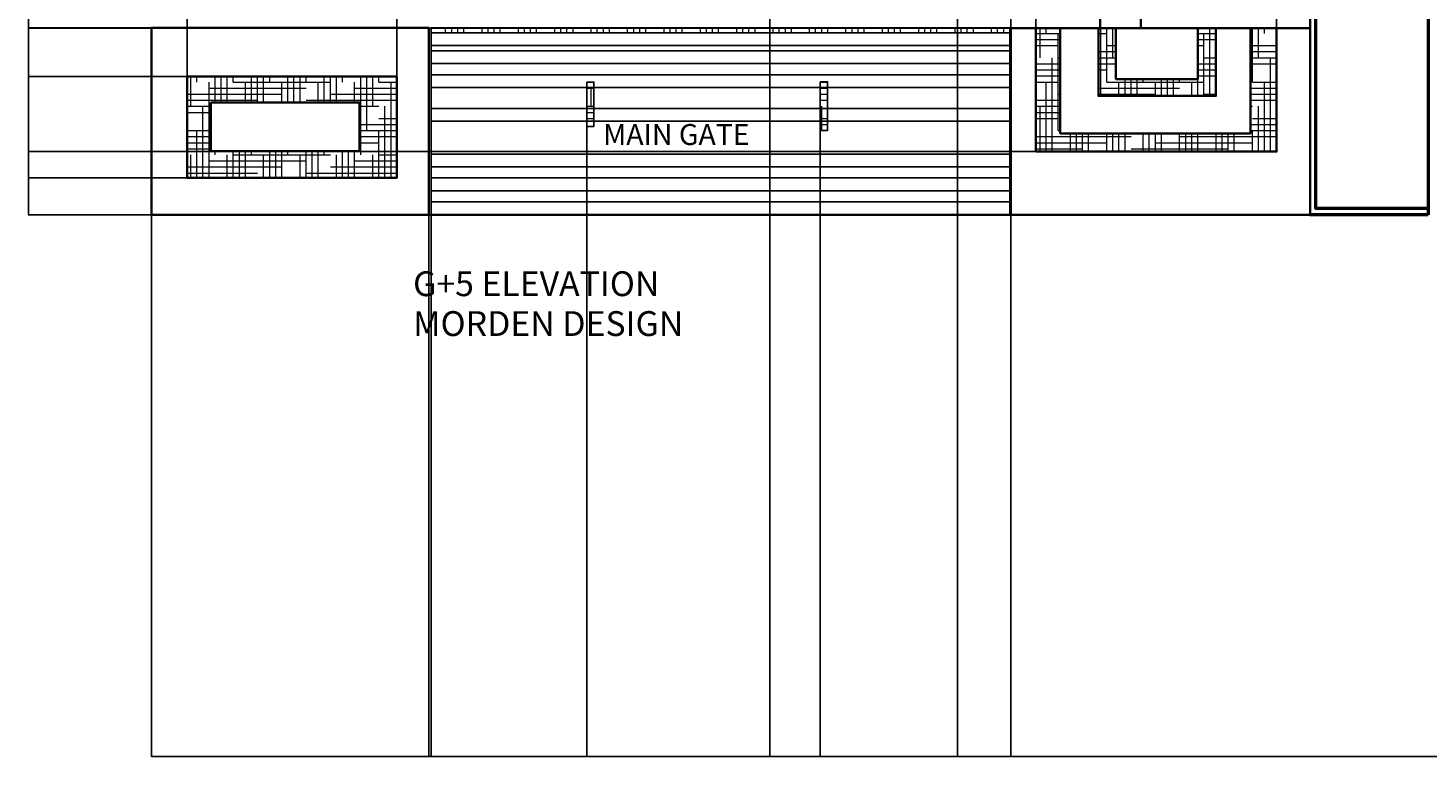
# Model space of a CAD drawing. Units: inches. Extents: x -97 to 1206, y -378 to 680.
# Tile 1 of 6: x -97 to 581, y -378 to -25. Entities that reach past the tile are written whole.
import ezdxf

# ---------------------------------------------------------------- set-up
doc = ezdxf.new("R2010")
doc.units = ezdxf.units.IN
doc.header["$MEASUREMENT"] = 0
for name, color, linetype, lineweight in [('A-ANNO-DIMS', 2, 'Continuous', 18), ('A-ANNO-TEXT', 7, 'Continuous', 25), ('A-DOOR', 3, 'Continuous', 25), ('A-ELEV', 7, 'Continuous', 35), ('A-ELEV-PATT', 252, 'Continuous', 13), ('A-WALL', 7, 'Continuous', 50)]:
    doc.layers.add(name, color=color, linetype=linetype, lineweight=lineweight)
doc.styles.get("Standard").update_dxf_attribs({"font": 'arial.ttf'})
doc.dimstyles.get("Standard").update_dxf_attribs({"dimtxt": 0.18, "dimasz": 0.18, "dimexe": 0.18, "dimexo": 0.0625, "dimgap": 0.09, "dimtad": 0, "dimtih": 1, "dimtoh": 1, "dimdec": 4, "dimzin": 0, "dimdsep": 46, "dimtxsty": 'Standard', "dimcen": 0.09, "dimadec": 0, "dimazin": 0, "dimtfac": 1, "dimtdec": 4, "dimtofl": 0, "dimtmove": 0, "dimatfit": 3, "dimfxl": 1, "dimtolj": 1, "dimtzin": 0, "dimarcsym": 0})

# ---------------------------------------------------------------- blocks, each defined once
blk = doc.blocks.new('*D11')
at = {"layer": 'A-ANNO-DIMS', "color": 0, "lineweight": -2, "transparency": 16777216}
for p, q in [((-36.91, -115.21), (-36.91, -377.59)), ((620.19, -115.21), (620.19, -377.59)), ((-36.73, -377.41), (291.26, -377.41)), ((620.01, -377.41), (292.02, -377.41))]:
    blk.add_line(p, q, dxfattribs=at)
at = {"layer": 'A-ANNO-DIMS', "color": 0, "transparency": 16777216}
for points in [[(-36.73, -377.38), (-36.73, -377.44), (-36.91, -377.41)], [(620.01, -377.38), (620.01, -377.44), (620.19, -377.41)]]:
    blk.add_solid(points, dxfattribs=at)
at = {"layer": 'Defpoints', "color": 0, "transparency": 16777216}
for p in [(-36.91, -115.14), (620.19, -115.14), (620.19, -377.41)]:
    blk.add_point(p, dxfattribs=at)
at = {"layer": 'A-ANNO-DIMS', "color": 0, "transparency": 16777216, "insert": (291.64, -377.41), "char_height": 0.18, "attachment_point": 5}
blk.add_mtext('\\A1;657.1', dxfattribs=at)
blk = doc.blocks.new('*D12')
at = {"layer": 'A-ANNO-DIMS', "color": 0, "lineweight": -2, "transparency": 16777216}
for p, q in [((43.86, 619.86), (-96.59, 619.86)), ((-96.41, 619.68), (-96.41, 252.54)), ((-96.41, -114.96), (-96.41, 252.17)), ((-36.97, -115.14), (-96.59, -115.14))]:
    blk.add_line(p, q, dxfattribs=at)
at = {"layer": 'A-ANNO-DIMS', "color": 0, "transparency": 16777216}
for points in [[(-96.44, 619.68), (-96.38, 619.68), (-96.41, 619.86)], [(-96.44, -114.96), (-96.38, -114.96), (-96.41, -115.14)]]:
    blk.add_solid(points, dxfattribs=at)
at = {"layer": 'Defpoints', "color": 0, "transparency": 16777216}
for p in [(43.93, 619.86), (-96.41, -115.14), (-36.91, -115.14)]:
    blk.add_point(p, dxfattribs=at)
at = {"layer": 'A-ANNO-DIMS', "color": 0, "transparency": 16777216, "insert": (-96.41, 252.36), "char_height": 0.18, "attachment_point": 5}
blk.add_mtext('\\A1;735', dxfattribs=at)
blk = doc.blocks.new('*D13')
at = {"layer": 'A-ANNO-DIMS', "color": 0, "lineweight": -2, "transparency": 16777216}
for p, q in [((46.86, 4.86), (-96.59, 4.86)), ((-96.41, 4.68), (-96.41, -54.96)), ((-96.41, -114.96), (-96.41, -55.33)), ((-36.97, -115.14), (-96.59, -115.14))]:
    blk.add_line(p, q, dxfattribs=at)
at = {"layer": 'A-ANNO-DIMS', "color": 0, "transparency": 16777216}
for points in [[(-96.44, 4.68), (-96.38, 4.68), (-96.41, 4.86)], [(-96.44, -114.96), (-96.38, -114.96), (-96.41, -115.14)]]:
    blk.add_solid(points, dxfattribs=at)
at = {"layer": 'Defpoints', "color": 0, "transparency": 16777216}
for p in [(46.93, 4.86), (-96.41, -115.14), (-36.91, -115.14)]:
    blk.add_point(p, dxfattribs=at)
at = {"layer": 'A-ANNO-DIMS', "color": 0, "transparency": 16777216, "insert": (-96.41, -55.14), "char_height": 0.18, "attachment_point": 5}
blk.add_mtext('\\A1;120', dxfattribs=at)
blk = doc.blocks.new('*D19')
at = {"layer": 'A-ANNO-DIMS', "color": 0, "lineweight": -2, "transparency": 16777216}
for p, q in [((-36.91, -115.21), (-36.91, -377.59)), ((97.45, -115.21), (97.45, -377.59)), ((-36.73, -377.41), (29.82, -377.41)), ((97.27, -377.41), (30.73, -377.41))]:
    blk.add_line(p, q, dxfattribs=at)
at = {"layer": 'A-ANNO-DIMS', "color": 0, "transparency": 16777216}
for points in [[(-36.73, -377.38), (-36.73, -377.44), (-36.91, -377.41)], [(97.27, -377.38), (97.27, -377.44), (97.45, -377.41)]]:
    blk.add_solid(points, dxfattribs=at)
at = {"layer": 'Defpoints', "color": 0, "transparency": 16777216}
for p in [(-36.91, -115.14), (97.45, -115.14), (97.45, -377.41)]:
    blk.add_point(p, dxfattribs=at)
at = {"layer": 'A-ANNO-DIMS', "color": 0, "transparency": 16777216, "insert": (30.27, -377.41), "char_height": 0.18, "attachment_point": 5}
blk.add_mtext('\\A1;134.35', dxfattribs=at)
blk = doc.blocks.new('*D20')
at = {"layer": 'A-ANNO-DIMS', "color": 0, "lineweight": -2, "transparency": 16777216}
for p, q in [((98.56, -115.21), (98.56, -377.59)), ((379.25, -115.21), (379.25, -377.59)), ((98.74, -377.41), (238.51, -377.41)), ((379.07, -377.41), (239.3, -377.41))]:
    blk.add_line(p, q, dxfattribs=at)
at = {"layer": 'A-ANNO-DIMS', "color": 0, "transparency": 16777216}
for points in [[(98.74, -377.38), (98.74, -377.44), (98.56, -377.41)], [(379.07, -377.38), (379.07, -377.44), (379.25, -377.41)]]:
    blk.add_solid(points, dxfattribs=at)
at = {"layer": 'Defpoints', "color": 0, "transparency": 16777216}
for p in [(98.56, -115.14), (379.25, -115.14), (379.25, -377.41)]:
    blk.add_point(p, dxfattribs=at)
at = {"layer": 'A-ANNO-DIMS', "color": 0, "transparency": 16777216, "insert": (238.91, -377.41), "char_height": 0.18, "attachment_point": 5}
blk.add_mtext('\\A1;280.7', dxfattribs=at)
blk = doc.blocks.new('*D21')
at = {"layer": 'A-ANNO-DIMS', "color": 0, "lineweight": -2, "transparency": 16777216}
for p, q in [((379.25, -24.78), (379.25, 679.54)), ((379.43, 679.36), (451.27, 679.36)), ((524.01, 679.36), (452.18, 679.36)), ((524.19, -24.78), (524.19, 679.54))]:
    blk.add_line(p, q, dxfattribs=at)
at = {"layer": 'A-ANNO-DIMS', "color": 0, "transparency": 16777216}
for points in [[(379.43, 679.39), (379.43, 679.33), (379.25, 679.36)], [(524.01, 679.39), (524.01, 679.33), (524.19, 679.36)]]:
    blk.add_solid(points, dxfattribs=at)
at = {"layer": 'Defpoints', "color": 0, "transparency": 16777216}
for p in [(524.19, 679.36), (379.25, -24.84), (524.19, -24.84)]:
    blk.add_point(p, dxfattribs=at)
at = {"layer": 'A-ANNO-DIMS', "color": 0, "transparency": 16777216, "insert": (451.72, 679.36), "char_height": 0.18, "attachment_point": 5}
blk.add_mtext('\\A1;144.94', dxfattribs=at)
blk = doc.blocks.new('*D35')
at = {"layer": 'A-ANNO-DIMS', "color": 0, "lineweight": -2, "transparency": 16777216}
for p, q in [((-36.97, -24.73), (-96.59, -24.73)), ((-96.41, -24.91), (-96.41, -69.75)), ((-96.41, -114.96), (-96.41, -70.12)), ((-36.97, -115.14), (-96.59, -115.14))]:
    blk.add_line(p, q, dxfattribs=at)
at = {"layer": 'A-ANNO-DIMS', "color": 0, "transparency": 16777216}
for points in [[(-96.44, -24.91), (-96.38, -24.91), (-96.41, -24.73)], [(-96.44, -114.96), (-96.38, -114.96), (-96.41, -115.14)]]:
    blk.add_solid(points, dxfattribs=at)
at = {"layer": 'Defpoints', "color": 0, "transparency": 16777216}
for p in [(-96.41, -24.73), (-36.91, -24.73), (-36.91, -115.14)]:
    blk.add_point(p, dxfattribs=at)
at = {"layer": 'A-ANNO-DIMS', "color": 0, "transparency": 16777216, "insert": (-96.41, -69.94), "char_height": 0.18, "attachment_point": 5}
blk.add_mtext('\\A1;90.42', dxfattribs=at)
blk = doc.blocks.new('*D36')
at = {"layer": 'A-ANNO-DIMS', "color": 0, "lineweight": -2, "transparency": 16777216}
for p, q in [((-19.68, -48.26), (-19.68, 679.54)), ((-19.5, 679.36), (30.69, 679.36)), ((81.65, 679.36), (31.46, 679.36)), ((81.83, -48.26), (81.83, 679.54))]:
    blk.add_line(p, q, dxfattribs=at)
at = {"layer": 'A-ANNO-DIMS', "color": 0, "transparency": 16777216}
for points in [[(-19.5, 679.39), (-19.5, 679.33), (-19.68, 679.36)], [(81.65, 679.39), (81.65, 679.33), (81.83, 679.36)]]:
    blk.add_solid(points, dxfattribs=at)
at = {"layer": 'Defpoints', "color": 0, "transparency": 16777216}
for p in [(81.83, 679.36), (-19.68, -48.33), (81.83, -48.33)]:
    blk.add_point(p, dxfattribs=at)
at = {"layer": 'A-ANNO-DIMS', "color": 0, "transparency": 16777216, "insert": (31.08, 679.36), "char_height": 0.18, "attachment_point": 5}
blk.add_mtext('\\A1;101.5', dxfattribs=at)
blk = doc.blocks.new('*D37')
at = {"layer": 'A-ANNO-DIMS', "color": 0, "lineweight": -2, "transparency": 16777216}
for p, q in [((-19.74, -48.33), (-96.59, -48.33)), ((-96.41, -48.51), (-96.41, -72.66)), ((-96.41, -97.18), (-96.41, -73.03)), ((-19.74, -97.36), (-96.59, -97.36))]:
    blk.add_line(p, q, dxfattribs=at)
at = {"layer": 'A-ANNO-DIMS', "color": 0, "transparency": 16777216}
for points in [[(-96.44, -48.51), (-96.38, -48.51), (-96.41, -48.33)], [(-96.44, -97.18), (-96.38, -97.18), (-96.41, -97.36)]]:
    blk.add_solid(points, dxfattribs=at)
at = {"layer": 'Defpoints', "color": 0, "transparency": 16777216}
for p in [(-19.68, -48.33), (-96.41, -97.36), (-19.68, -97.36)]:
    blk.add_point(p, dxfattribs=at)
at = {"layer": 'A-ANNO-DIMS', "color": 0, "transparency": 16777216, "insert": (-96.41, -72.85), "char_height": 0.18, "attachment_point": 5}
blk.add_mtext('\\A1;49.04', dxfattribs=at)
blk = doc.blocks.new('*D38')
at = {"layer": 'A-ANNO-DIMS', "color": 0, "lineweight": -2, "transparency": 16777216}
for p, q in [((391.36, -84.5), (391.36, 679.54)), ((391.54, 679.36), (449.18, 679.36)), ((507.74, 679.36), (450.1, 679.36)), ((507.92, -84.5), (507.92, 679.54))]:
    blk.add_line(p, q, dxfattribs=at)
at = {"layer": 'A-ANNO-DIMS', "color": 0, "transparency": 16777216}
for points in [[(391.54, 679.39), (391.54, 679.33), (391.36, 679.36)], [(507.74, 679.39), (507.74, 679.33), (507.92, 679.36)]]:
    blk.add_solid(points, dxfattribs=at)
at = {"layer": 'Defpoints', "color": 0, "transparency": 16777216}
for p in [(507.92, 679.36), (391.36, -84.57), (507.92, -84.57)]:
    blk.add_point(p, dxfattribs=at)
at = {"layer": 'A-ANNO-DIMS', "color": 0, "transparency": 16777216, "insert": (449.64, 679.36), "char_height": 0.18, "attachment_point": 5}
blk.add_mtext('\\A1;116.56', dxfattribs=at)
blk = doc.blocks.new('*D39')
at = {"layer": 'A-ANNO-DIMS', "color": 0, "lineweight": -2, "transparency": 16777216}
for p, q in [((391.3, -24.84), (-96.59, -24.84)), ((-96.41, -25.02), (-96.41, -54.52)), ((-96.41, -84.39), (-96.41, -54.89)), ((391.3, -84.57), (-96.59, -84.57))]:
    blk.add_line(p, q, dxfattribs=at)
at = {"layer": 'A-ANNO-DIMS', "color": 0, "transparency": 16777216}
for points in [[(-96.44, -25.02), (-96.38, -25.02), (-96.41, -24.84)], [(-96.44, -84.39), (-96.38, -84.39), (-96.41, -84.57)]]:
    blk.add_solid(points, dxfattribs=at)
at = {"layer": 'Defpoints', "color": 0, "transparency": 16777216}
for p in [(391.36, -24.84), (-96.41, -84.57), (391.36, -84.57)]:
    blk.add_point(p, dxfattribs=at)
at = {"layer": 'A-ANNO-DIMS', "color": 0, "transparency": 16777216, "insert": (-96.41, -54.7), "char_height": 0.18, "attachment_point": 5}
blk.add_mtext('\\A1;59.72', dxfattribs=at)
blk = doc.blocks.new('*D43')
at = {"layer": 'A-ANNO-DIMS', "color": 0, "lineweight": -2, "transparency": 16777216}
for p, q in [((262.49, 49.82), (262.49, -377.59)), ((353.38, 49.82), (353.38, -377.59)), ((262.67, -377.41), (307.54, -377.41)), ((353.2, -377.41), (308.33, -377.41))]:
    blk.add_line(p, q, dxfattribs=at)
at = {"layer": 'A-ANNO-DIMS', "color": 0, "transparency": 16777216}
for points in [[(262.67, -377.38), (262.67, -377.44), (262.49, -377.41)], [(353.2, -377.38), (353.2, -377.44), (353.38, -377.41)]]:
    blk.add_solid(points, dxfattribs=at)
at = {"layer": 'Defpoints', "color": 0, "transparency": 16777216}
for p in [(262.49, 49.88), (353.38, 49.88), (353.38, -377.41)]:
    blk.add_point(p, dxfattribs=at)
at = {"layer": 'A-ANNO-DIMS', "color": 0, "transparency": 16777216, "insert": (307.94, -377.41), "char_height": 0.18, "attachment_point": 5}
blk.add_mtext('\\A1;90.88', dxfattribs=at)
blk = doc.blocks.new('*D49')
at = {"layer": 'A-ANNO-DIMS', "color": 0, "lineweight": -2, "transparency": 16777216}
for p, q in [((98.56, -70), (98.56, -377.59)), ((173.91, -72.5), (173.91, -377.59)), ((98.74, -377.41), (135.84, -377.41)), ((173.73, -377.41), (136.63, -377.41))]:
    blk.add_line(p, q, dxfattribs=at)
at = {"layer": 'A-ANNO-DIMS', "color": 0, "transparency": 16777216}
for points in [[(98.74, -377.38), (98.74, -377.44), (98.56, -377.41)], [(173.73, -377.38), (173.73, -377.44), (173.91, -377.41)]]:
    blk.add_solid(points, dxfattribs=at)
at = {"layer": 'Defpoints', "color": 0, "transparency": 16777216}
for p in [(98.56, -69.94), (173.91, -72.44), (173.91, -377.41)]:
    blk.add_point(p, dxfattribs=at)
at = {"layer": 'A-ANNO-DIMS', "color": 0, "transparency": 16777216, "insert": (136.23, -377.41), "char_height": 0.18, "attachment_point": 5}
blk.add_mtext('\\A1;75.35', dxfattribs=at)
blk = doc.blocks.new('*D50')
at = {"layer": 'A-ANNO-DIMS', "color": 0, "lineweight": -2, "transparency": 16777216}
for p, q in [((173.91, -72.5), (173.91, -377.59)), ((286.82, -74.44), (286.82, -377.59)), ((174.09, -377.41), (229.98, -377.41)), ((286.64, -377.41), (230.75, -377.41))]:
    blk.add_line(p, q, dxfattribs=at)
at = {"layer": 'A-ANNO-DIMS', "color": 0, "transparency": 16777216}
for points in [[(174.09, -377.38), (174.09, -377.44), (173.91, -377.41)], [(286.64, -377.38), (286.64, -377.44), (286.82, -377.41)]]:
    blk.add_solid(points, dxfattribs=at)
at = {"layer": 'Defpoints', "color": 0, "transparency": 16777216}
for p in [(173.91, -72.44), (286.82, -74.38), (286.82, -377.41)]:
    blk.add_point(p, dxfattribs=at)
at = {"layer": 'A-ANNO-DIMS', "color": 0, "transparency": 16777216, "insert": (230.36, -377.41), "char_height": 0.18, "attachment_point": 5}
blk.add_mtext('\\A1;112.9', dxfattribs=at)

msp = doc.modelspace()

# ---------------------------------------------------------------- hatches: boundary and pattern name
at = {"layer": 'A-ELEV-PATT'}
h = msp.add_hatch(dxfattribs=at)
h.set_pattern_fill('HOUND', color=256, scale=47)
h.set_pattern_definition([(0, (-208.809, -191.922), (11.75, 2.9375), [47, -23.5]), (90, (-208.809, -191.922), (-2.9375, -11.75), [47, -23.5])])
h.paths.add_polyline_path([(81.8295, -48.3264), (-19.6789, -48.3264), (-19.6789, -97.3647), (81.8295, -97.3647)])
h.paths.add_polyline_path([(-8.2183, -60.8667), (63.8199, -60.8667), (63.8199, -84.3116), (-8.2183, -84.3116)], flags=16)
h.paths.add_polyline_path([(403.1688, -24.8426), (391.3618, -24.8426), (391.3618, -84.5669), (507.9182, -84.5669), (507.9182, -24.8426), (495.2029, -24.8426), (495.2029, -75.7956), (403.1688, -75.7956)])
h.paths.add_polyline_path([(430.113, -24.8426), (421.6362, -24.8426), (421.6362, -57.6481), (478.552, -57.6481), (478.552, -24.8426), (469.7725, -24.8426), (469.7725, -49.4817), (430.113, -49.4817)], flags=17)
h.paths.add_polyline_path([(378.6527, -24.7259), (98.5594, -24.7259), (98.5594, -27.0887), (378.6527, -27.0887)])
h.paths.add_polyline_path([(177.3114, -53.6191), (173.9058, -53.6191), (173.9058, -63.7423), (177.3114, -63.7423)])
h.paths.add_polyline_path([(177.3114, -63.7423), (173.9058, -63.7423), (173.9058, -69.9353), (177.3114, -69.9353)])
h.paths.add_polyline_path([(290.4371, -69.9353), (286.815, -69.9353), (286.815, -74.3824), (290.4371, -74.3824)])
h.paths.add_polyline_path([(290.4371, -63.7423), (286.815, -63.7423), (286.815, -69.9353), (290.4371, -69.9353)])
h.paths.add_polyline_path([(290.4371, -53.6191), (286.815, -53.6191), (286.815, -63.7423), (290.4371, -63.7423)])
h.paths.add_polyline_path([(290.4371, -50.7545), (286.815, -50.7545), (286.815, -53.6191), (290.4371, -53.6191)])

# ---------------------------------------------------------------- linework, layer by layer
at = {"layer": 'A-DOOR'}
for points in [[(98.5594, -24.7259), (378.6527, -24.7259), (378.6527, -115.1448), (98.5594, -115.1448)], [(98.5594, -27.0887), (379.2519, -27.0887), (379.2519, -33.2816), (98.5594, -33.2816)], [(98.5594, -35.7509), (379.2519, -35.7509), (379.2519, -41.9439), (98.5594, -41.9439)], [(98.5594, -47.4262), (379.2519, -47.4262), (379.2519, -53.6191), (98.5594, -53.6191)], [(173.9058, -50.964), (177.3114, -50.964), (177.3114, -72.4413), (173.9058, -72.4413)], [(286.815, -50.7545), (290.4371, -50.7545), (290.4371, -74.3824), (286.815, -74.3824)], [(98.5594, -63.7423), (379.2519, -63.7423), (379.2519, -69.9353), (98.5594, -69.9353)], [(98.5594, -85.8004), (379.2519, -85.8004), (379.2519, -91.9933), (98.5594, -91.9933)], [(98.5594, -97.3647), (379.2519, -97.3647), (379.2519, -103.5577), (98.5594, -103.5577)], [(98.5594, -108.9518), (379.2519, -108.9518), (379.2519, -115.1448), (98.5594, -115.1448)]]:
    msp.add_lwpolyline(points, close=True, dxfattribs=at)
at = {"layer": 'A-ELEV'}
msp.add_lwpolyline([(46.9261, 4.8552), (524.19, 4.8552), (524.19, -115.1448), (43.9261, -115.1448)], dxfattribs=at)
for points in [[(442.2146, -24.8426), (422.4455, -24.8426), (422.4455, 4.8552), (442.2146, 4.8552)], [(-36.9051, -24.7259), (97.4484, -24.7259), (97.4484, -115.1448), (-36.9051, -115.1448)], [(379.2519, -24.8426), (524.19, -24.8426), (524.19, -115.1448), (379.2519, -115.1448)], [(391.3618, -24.8426), (507.9182, -24.8426), (507.9182, -84.5669), (391.3618, -84.5669)], [(403.1688, -24.8426), (495.2029, -24.8426), (495.2029, -75.7956), (403.1688, -75.7956)], [(421.6362, -24.8426), (478.552, -24.8426), (478.552, -57.6481), (421.6362, -57.6481)], [(430.113, -24.8426), (469.7725, -24.8426), (469.7725, -49.4817), (430.113, -49.4817)], [(-19.6789, -48.3264), (81.8295, -48.3264), (81.8295, -97.3647), (-19.6789, -97.3647)], [(-8.2183, -60.8667), (63.8199, -60.8667), (63.8199, -84.3116), (-8.2183, -84.3116)]]:
    msp.add_lwpolyline(points, close=True, dxfattribs=at)
at = {"layer": 'A-WALL'}
for points in [[(581.2095, 619.8552), (581.2095, -115.1448)], [(581.2095, -112.1448), (526.9261, -112.1448), (526.9261, 616.8552), (581.2095, 616.8552)], [(581.2095, -115.1448), (523.9261, -115.1448)]]:
    msp.add_lwpolyline(points, dxfattribs=at)

# ---------------------------------------------------------------- texts
at = {"layer": 'A-ANNO-TEXT'}
for s, height, p in [('MAIN GATE', 10.10681, (181.7879, -81.3868)), ('G+5 ELEVATION ', 12, (89.7601, -154.5495)), ('MORDEN DESIGN', 12, (89.7601, -173.8264))]:
    msp.add_text(s, height=height, dxfattribs=at).set_placement(p)

# ---------------------------------------------------------------- dimensions: what is measured, and where the dimension line sits
at = {"layer": 'A-ANNO-DIMS'}
for base, p1, p2, override, picture, middle in [((81.8295, 679.3552), (-19.6789, -48.3264), (81.8295, -48.3264), {"dimdec": 1, "dimlfac": 1, "dimrnd": 0, "dimzin": 0, "dimdsep": 46, "dimlunit": 2}, '*D36', (31.0753, 679.3552)), ((524.19, 679.3552), (379.2519, -24.8426), (524.19, -24.8426), {"dimdec": 2, "dimlfac": 1, "dimrnd": 0, "dimzin": 0, "dimdsep": 46, "dimlunit": 2}, '*D21', (451.721, 679.3552)), ((507.9182, 679.3552), (391.3618, -84.5669), (507.9182, -84.5669), {"dimdec": 2, "dimlfac": 1, "dimrnd": 0, "dimzin": 0, "dimdsep": 46, "dimlunit": 2}, '*D38', (449.64, 679.3552)), ((353.3784, -377.4132), (262.4936, 49.8815), (353.3784, 49.8815), {"dimdec": 2, "dimlfac": 1, "dimrnd": 0, "dimzin": 0, "dimdsep": 46, "dimlunit": 2}, '*D43', (307.936, -377.4132)), ((173.9058, -377.4132), (98.5594, -69.9353), (173.9058, -72.4413), {"dimdec": 2, "dimlfac": 1, "dimrnd": 0, "dimzin": 0, "dimdsep": 46, "dimlunit": 2}, '*D49', (136.2326, -377.4132)), ((286.815, -377.4132), (173.9058, -72.4413), (286.815, -74.3824), {"dimdec": 1, "dimlfac": 1, "dimrnd": 0, "dimzin": 0, "dimdsep": 46, "dimlunit": 2}, '*D50', (230.3604, -377.4132)), ((620.1851, -377.4132), (-36.9051, -115.1448), (620.1851, -115.1448), {"dimdec": 1, "dimlfac": 1, "dimrnd": 0, "dimzin": 0, "dimdsep": 46, "dimlunit": 2}, '*D11', (291.64, -377.4132)), ((97.4484, -377.4132), (-36.9051, -115.1448), (97.4484, -115.1448), {"dimdec": 2, "dimlfac": 1, "dimrnd": 0, "dimzin": 0, "dimdsep": 46, "dimlunit": 2}, '*D19', (30.2716, -377.4132)), ((379.2519, -377.4132), (98.5594, -115.1448), (379.2519, -115.1448), {"dimdec": 1, "dimlfac": 1, "dimrnd": 0, "dimzin": 0, "dimdsep": 46, "dimlunit": 2}, '*D20', (238.9057, -377.4132))]:
    dim = msp.add_linear_dim(base=base, p1=p1, p2=p2, dimstyle='Standard', override=override, dxfattribs=at)
    dim.commit()
    dim.dimension.update_dxf_attribs({"geometry": picture, "text_midpoint": middle})
for base, p1, p2, override, picture, middle in [((-96.4051, -115.1448), (43.9261, 619.8552), (-36.9051, -115.1448), {"dimdec": 0, "dimlfac": 1, "dimrnd": 0, "dimzin": 0, "dimdsep": 46, "dimlunit": 2}, '*D12', (-96.4051, 252.3552)), ((-96.4051, -115.1448), (46.9261, 4.8552), (-36.9051, -115.1448), {"dimdec": 0, "dimlfac": 1, "dimrnd": 0, "dimzin": 0, "dimdsep": 46, "dimlunit": 2}, '*D13', (-96.4051, -55.1448)), ((-96.4051, -24.7259), (-36.9051, -115.1448), (-36.9051, -24.7259), {"dimdec": 2, "dimlfac": 1, "dimrnd": 0, "dimzin": 0, "dimdsep": 46, "dimlunit": 2}, '*D35', (-96.4051, -69.9353)), ((-96.4051, -84.5669), (391.3618, -24.8426), (391.3618, -84.5669), {"dimdec": 2, "dimlfac": 1, "dimrnd": 0, "dimzin": 0, "dimdsep": 46, "dimlunit": 2}, '*D39', (-96.4051, -54.7048)), ((-96.4051, -97.3647), (-19.6789, -48.3264), (-19.6789, -97.3647), {"dimdec": 2, "dimlfac": 1, "dimrnd": 0, "dimzin": 0, "dimdsep": 46, "dimlunit": 2}, '*D37', (-96.4051, -72.8456))]:
    dim = msp.add_linear_dim(base=base, p1=p1, p2=p2, angle=90, dimstyle='Standard', override=override, dxfattribs=at)
    dim.commit()
    dim.dimension.update_dxf_attribs({"geometry": picture, "text_midpoint": middle})

doc.saveas('drawing.dxf')
